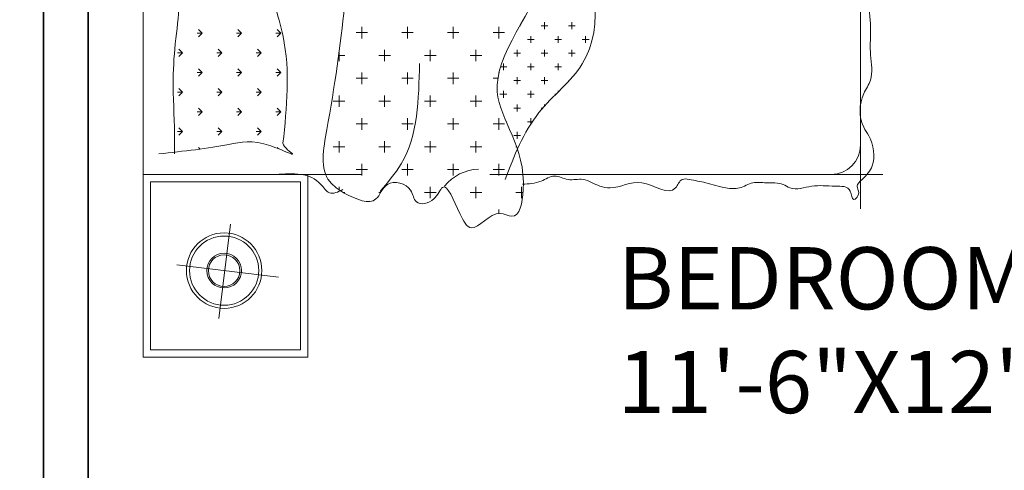
# Model space of a CAD drawing. Units: inches. Extents: x 3731 to 4318, y 1310 to 2388.
# Tile 35 of 57: x 3833 to 3943, y 2192 to 2243. Entities that reach past the tile are written whole.
import ezdxf

# ---------------------------------------------------------------- set-up
doc = ezdxf.new("R2010")
doc.units = ezdxf.units.IN
for name, color, linetype, lineweight in [('A-ANNO-DIMS', 2, 'Continuous', 18), ('A-AREA-IDEN', 7, 'Continuous', 18), ('A-FURN', 8, 'Continuous', 13), ('A-WALL', 7, 'Continuous', 35)]:
    doc.layers.add(name, color=color, linetype=linetype, lineweight=lineweight)
doc.styles.get("Standard").update_dxf_attribs({"font": 'arial.ttf'})
doc.dimstyles.get("Standard").update_dxf_attribs({"dimtxt": 0.18, "dimasz": 0.18, "dimexe": 0.18, "dimexo": 0.0625, "dimgap": 0.09, "dimtad": 0, "dimtih": 1, "dimtoh": 1, "dimdec": 4, "dimzin": 0, "dimdsep": 46, "dimtxsty": 'Standard', "dimcen": 0.09, "dimadec": 0, "dimazin": 0, "dimtfac": 1, "dimtdec": 4, "dimtofl": 0, "dimtmove": 0, "dimatfit": 3, "dimfxl": 1, "dimtolj": 1, "dimtzin": 0, "dimarcsym": 0})

# ---------------------------------------------------------------- blocks, each defined once
blk = doc.blocks.new('A$C200C7901')
for p, q in [((0, 1.8834), (0, 2.3334)), ((0.5, 2.3334), (0, 2.3334)), ((0.5, 2.3334), (0.5, 1.7369)), ((0.5, 2.3334), (0.5, 1.7369)), ((0.5, 2.3334), (2, 2.3334)), ((0.5701, 1.9635), (0.5733, 1.9666)), ((0.5701, 1.9635), (0.5733, 1.9666)), ((0.5, 1.8834), (0, 1.8834)), ((0.4504, 1.782), (0.4504, 1.7863)), ((0.4504, 1.782), (0.4504, 1.7863)), ((0.458, 1.7977), (0.466, 1.7977)), ((0.458, 1.7977), (0.466, 1.7977)), ((0.4504, 1.6834), (0.4504, 1.6883)), ((0.4504, 1.6834), (0.4504, 1.6883)), ((0.4656, 1.6727), (0.466, 1.6727)), ((0.4656, 1.6727), (0.466, 1.6727)), ((0.5597, 1.6727), (0.591, 1.6727)), ((0.5597, 1.6727), (0.591, 1.6727)), ((0.4504, 1.532), (0.4504, 1.5633)), ((0.4347, 1.5477), (0.466, 1.5477)), ((0.6847, 1.5477), (0.716, 1.5477)), ((0.4347, 1.4227), (0.466, 1.4227)), ((0.5, 1.3845), (0.5, 0.3086)), ((0.3931, 1.3602), (0.4035, 1.3602)), ((0.3931, 1.3602), (0.4035, 1.3602)), ((0.4972, 1.3602), (0.5285, 1.3602)), ((0.4972, 1.3602), (0.5285, 1.3602)), ((0.4347, 1.2977), (0.466, 1.2977)), ((0.4347, 1.2977), (0.466, 1.2977)), ((0.4504, 1.2936), (0.4504, 1.3133)), ((0.4504, 1.2936), (0.4504, 1.3133)), ((0.4061, 0.3703), (2.0386, 0.3703))]:
    blk.add_line(p, q)
at = {"linetype": 'ByBlock'}
for p, q in [((0.02, 1.9034), (0.02, 2.3134)), ((0.48, 2.3134), (0.02, 2.3134)), ((0.48, 1.9034), (0.48, 2.3134)), ((0.2524, 2.2412), (0.2186, 1.9635)), ((0.6171, 2.2259), (0.6171, 2.2402)), ((0.6171, 2.2259), (0.6171, 2.2402)), ((0.7249, 2.2259), (0.7249, 2.2402)), ((0.7249, 2.2259), (0.7249, 2.2402)), ((0.8326, 2.2259), (0.8326, 2.2402)), ((0.8326, 2.2259), (0.8326, 2.2402)), ((0.6171, 2.2259), (0.607, 2.236)), ((0.6171, 2.2259), (0.607, 2.236)), ((0.6171, 2.2259), (0.6272, 2.236)), ((0.6171, 2.2259), (0.6272, 2.236)), ((0.7249, 2.2259), (0.7148, 2.236)), ((0.7249, 2.2259), (0.7148, 2.236)), ((0.7249, 2.2259), (0.735, 2.236)), ((0.7249, 2.2259), (0.735, 2.236)), ((0.8326, 2.2259), (0.8225, 2.236)), ((0.8326, 2.2259), (0.8225, 2.236)), ((0.8326, 2.2259), (0.8427, 2.236)), ((0.8326, 2.2259), (0.8427, 2.236)), ((0.671, 2.172), (0.671, 2.1863)), ((0.671, 2.172), (0.671, 2.1863)), ((0.7787, 2.172), (0.7787, 2.1863)), ((0.7787, 2.172), (0.7787, 2.1863)), ((0.8865, 2.172), (0.8865, 2.1863)), ((0.8865, 2.172), (0.8865, 2.1863)), ((0.5692, 2.178), (0.5733, 2.1822)), ((0.5692, 2.178), (0.5733, 2.1822)), ((0.671, 2.1721), (0.6609, 2.1822)), ((0.671, 2.1721), (0.6609, 2.1822)), ((0.671, 2.1721), (0.6811, 2.1822)), ((0.671, 2.1721), (0.6811, 2.1822)), ((0.7787, 2.1721), (0.7686, 2.1822)), ((0.7787, 2.1721), (0.7686, 2.1822)), ((0.7787, 2.1721), (0.7889, 2.1822)), ((0.7787, 2.1721), (0.7889, 2.1822)), ((0.8865, 2.1721), (0.8764, 2.1822)), ((0.8865, 2.1721), (0.8764, 2.1822)), ((0.8865, 2.1721), (0.8966, 2.1822)), ((0.8865, 2.1721), (0.8966, 2.1822)), ((0.6171, 2.1182), (0.6171, 2.1325)), ((0.6171, 2.1182), (0.6171, 2.1325)), ((0.7249, 2.1182), (0.7249, 2.1325)), ((0.7249, 2.1182), (0.7249, 2.1325)), ((0.8326, 2.1182), (0.8326, 2.1325)), ((0.8326, 2.1182), (0.8326, 2.1325)), ((0.3641, 2.0951), (0.1061, 2.1268)), ((0.6171, 2.1182), (0.607, 2.1283)), ((0.6171, 2.1182), (0.607, 2.1283)), ((0.6171, 2.1182), (0.6272, 2.1283)), ((0.6171, 2.1182), (0.6272, 2.1283)), ((0.7249, 2.1182), (0.7148, 2.1283)), ((0.7249, 2.1182), (0.7148, 2.1283)), ((0.7249, 2.1182), (0.735, 2.1283)), ((0.7249, 2.1182), (0.735, 2.1283)), ((0.8326, 2.1182), (0.8225, 2.1283)), ((0.8326, 2.1182), (0.8225, 2.1283)), ((0.8326, 2.1182), (0.8427, 2.1283)), ((0.8326, 2.1182), (0.8427, 2.1283)), ((0.671, 2.0643), (0.671, 2.0786)), ((0.671, 2.0643), (0.671, 2.0786)), ((0.7787, 2.0643), (0.7787, 2.0786)), ((0.7787, 2.0643), (0.7787, 2.0786)), ((0.8865, 2.0643), (0.8865, 2.0786)), ((0.8865, 2.0643), (0.8865, 2.0786)), ((0.671, 2.0643), (0.6609, 2.0744)), ((0.671, 2.0643), (0.6609, 2.0744)), ((0.671, 2.0643), (0.6811, 2.0744)), ((0.671, 2.0643), (0.6811, 2.0744)), ((0.7787, 2.0643), (0.7686, 2.0744)), ((0.7787, 2.0643), (0.7686, 2.0744)), ((0.7787, 2.0643), (0.7889, 2.0744)), ((0.7787, 2.0643), (0.7889, 2.0744)), ((0.8865, 2.0643), (0.8764, 2.0744)), ((0.8865, 2.0643), (0.8764, 2.0744)), ((0.8865, 2.0643), (0.8966, 2.0744)), ((0.8865, 2.0643), (0.8966, 2.0744)), ((0.6171, 2.0104), (0.6171, 2.0247)), ((0.6171, 2.0104), (0.6171, 2.0247)), ((0.7249, 2.0104), (0.7249, 2.0247)), ((0.7249, 2.0104), (0.7249, 2.0247)), ((0.8326, 2.0104), (0.8326, 2.0247)), ((0.8326, 2.0104), (0.8326, 2.0247)), ((0.6171, 2.0104), (0.607, 2.0205)), ((0.6171, 2.0104), (0.607, 2.0205)), ((0.6171, 2.0104), (0.6272, 2.0205)), ((0.6171, 2.0104), (0.6272, 2.0205)), ((0.7249, 2.0104), (0.7148, 2.0205)), ((0.7249, 2.0104), (0.7148, 2.0205)), ((0.7249, 2.0104), (0.735, 2.0205)), ((0.7249, 2.0104), (0.735, 2.0205)), ((0.8326, 2.0104), (0.8225, 2.0205)), ((0.8326, 2.0104), (0.8225, 2.0205)), ((0.8326, 2.0104), (0.8427, 2.0205)), ((0.8326, 2.0104), (0.8427, 2.0205)), ((0.671, 1.9565), (0.671, 1.9708)), ((0.671, 1.9565), (0.671, 1.9708)), ((0.7787, 1.9565), (0.7787, 1.9708)), ((0.7787, 1.9565), (0.7787, 1.9708)), ((0.8865, 1.9565), (0.8865, 1.9708)), ((0.8865, 1.9565), (0.8865, 1.9708)), ((0.671, 1.9565), (0.6609, 1.9666)), ((0.671, 1.9565), (0.6609, 1.9666)), ((0.671, 1.9565), (0.6811, 1.9666)), ((0.671, 1.9565), (0.6811, 1.9666)), ((0.7787, 1.9565), (0.7686, 1.9666)), ((0.7787, 1.9565), (0.7686, 1.9666)), ((0.7787, 1.9565), (0.7889, 1.9666)), ((0.7787, 1.9565), (0.7889, 1.9666)), ((0.8865, 1.9565), (0.8764, 1.9666)), ((0.8865, 1.9565), (0.8764, 1.9666)), ((0.8865, 1.9565), (0.8966, 1.9666)), ((0.8865, 1.9565), (0.8966, 1.9666)), ((0.48, 1.9034), (0.02, 1.9034)), ((0.5754, 1.782), (0.5754, 1.8133)), ((0.5754, 1.782), (0.5754, 1.8133)), ((0.7004, 1.782), (0.7004, 1.8133)), ((0.7004, 1.782), (0.7004, 1.8133)), ((0.5597, 1.7977), (0.591, 1.7977)), ((0.5597, 1.7977), (0.591, 1.7977)), ((0.6847, 1.7977), (0.716, 1.7977)), ((0.6847, 1.7977), (0.716, 1.7977)), ((0.8097, 1.7977), (0.8331, 1.7977)), ((0.8097, 1.7977), (0.8331, 1.7977)), ((0.8254, 1.782), (0.8254, 1.7987)), ((0.8254, 1.782), (0.8254, 1.7987)), ((0.4972, 1.7352), (0.5285, 1.7352)), ((0.4972, 1.7352), (0.5285, 1.7352)), ((0.5129, 1.7195), (0.5129, 1.7508)), ((0.5129, 1.7195), (0.5129, 1.7508)), ((0.6222, 1.7352), (0.6535, 1.7352)), ((0.6222, 1.7352), (0.6535, 1.7352)), ((0.6379, 1.7195), (0.6379, 1.7508)), ((0.6379, 1.7195), (0.6379, 1.7508)), ((0.7472, 1.7352), (0.7785, 1.7352)), ((0.7472, 1.7352), (0.7785, 1.7352)), ((0.7629, 1.7195), (0.7629, 1.7508)), ((0.7629, 1.7195), (0.7629, 1.7508)), ((0.8722, 1.7352), (0.9035, 1.7352)), ((0.8722, 1.7352), (0.9035, 1.7352)), ((0.8879, 1.7195), (0.8879, 1.7508)), ((0.8879, 1.7195), (0.8879, 1.7508)), ((0.5754, 1.657), (0.5754, 1.6883)), ((0.5754, 1.657), (0.5754, 1.6883)), ((0.6847, 1.6727), (0.716, 1.6727)), ((0.6847, 1.6727), (0.716, 1.6727)), ((0.7004, 1.657), (0.7004, 1.6883)), ((0.7004, 1.657), (0.7004, 1.6883)), ((0.8097, 1.6727), (0.841, 1.6727)), ((0.8097, 1.6727), (0.841, 1.6727)), ((0.8254, 1.657), (0.8254, 1.6883)), ((0.8254, 1.657), (0.8254, 1.6883)), ((0.5129, 1.5945), (0.5129, 1.6258)), ((0.5129, 1.5945), (0.5129, 1.6258)), ((0.6379, 1.5945), (0.6379, 1.6258)), ((0.6379, 1.5945), (0.6379, 1.6258)), ((0.7629, 1.5945), (0.7629, 1.6258)), ((0.7629, 1.5945), (0.7629, 1.6258)), ((0.8879, 1.5945), (0.8879, 1.6258)), ((0.8879, 1.5945), (0.8879, 1.6258)), ((0.4972, 1.6102), (0.5285, 1.6102)), ((0.4972, 1.6102), (0.5285, 1.6102)), ((0.6222, 1.6102), (0.6535, 1.6102)), ((0.6222, 1.6102), (0.6535, 1.6102)), ((0.7472, 1.6102), (0.7785, 1.6102)), ((0.7472, 1.6102), (0.7785, 1.6102)), ((0.8722, 1.6102), (0.9035, 1.6102)), ((0.8722, 1.6102), (0.9035, 1.6102)), ((0.4504, 1.532), (0.4504, 1.5633)), ((0.5754, 1.532), (0.5754, 1.5633)), ((0.5754, 1.532), (0.5754, 1.5633)), ((0.7004, 1.532), (0.7004, 1.5633)), ((0.7004, 1.532), (0.7004, 1.5633)), ((0.8254, 1.532), (0.8254, 1.5633)), ((0.8254, 1.532), (0.8254, 1.5633)), ((0.4347, 1.5477), (0.466, 1.5477)), ((0.5597, 1.5477), (0.591, 1.5477)), ((0.5597, 1.5477), (0.591, 1.5477)), ((0.6847, 1.5477), (0.716, 1.5477)), ((0.8097, 1.5477), (0.841, 1.5477)), ((0.8097, 1.5477), (0.841, 1.5477)), ((0.4972, 1.4852), (0.5285, 1.4852)), ((0.4972, 1.4852), (0.5285, 1.4852)), ((0.5129, 1.4695), (0.5129, 1.5008)), ((0.5129, 1.4695), (0.5129, 1.5008)), ((0.6222, 1.4852), (0.6535, 1.4852)), ((0.6222, 1.4852), (0.6535, 1.4852)), ((0.6379, 1.4695), (0.6379, 1.5008)), ((0.6379, 1.4695), (0.6379, 1.5008)), ((0.7472, 1.4852), (0.7785, 1.4852)), ((0.7472, 1.4852), (0.7785, 1.4852)), ((0.7629, 1.4695), (0.7629, 1.5008)), ((0.7629, 1.4695), (0.7629, 1.5008)), ((0.8722, 1.4852), (0.9035, 1.4852)), ((0.8722, 1.4852), (0.9035, 1.4852)), ((0.8879, 1.4695), (0.8879, 1.5008)), ((0.8879, 1.4695), (0.8879, 1.5008)), ((0.4504, 1.407), (0.4504, 1.4383)), ((0.4504, 1.407), (0.4504, 1.4383)), ((0.5754, 1.407), (0.5754, 1.4383)), ((0.5754, 1.407), (0.5754, 1.4383)), ((0.7004, 1.407), (0.7004, 1.4383)), ((0.7004, 1.407), (0.7004, 1.4383)), ((0.8254, 1.407), (0.8254, 1.4383)), ((0.8254, 1.407), (0.8254, 1.4383)), ((0.4347, 1.4227), (0.466, 1.4227)), ((0.5597, 1.4227), (0.591, 1.4227)), ((0.5597, 1.4227), (0.591, 1.4227)), ((0.6847, 1.4227), (0.716, 1.4227)), ((0.6847, 1.4227), (0.716, 1.4227)), ((0.8097, 1.4227), (0.841, 1.4227)), ((0.8097, 1.4227), (0.841, 1.4227)), ((0.5129, 1.3445), (0.5129, 1.3758)), ((0.5129, 1.3445), (0.5129, 1.3758)), ((0.6379, 1.3445), (0.6379, 1.3758)), ((0.6379, 1.3445), (0.6379, 1.3758)), ((0.7629, 1.3627), (0.7629, 1.3758)), ((0.7629, 1.3627), (0.7629, 1.3758)), ((0.8879, 1.3445), (0.8879, 1.3758)), ((0.8879, 1.3445), (0.8879, 1.3758)), ((0.6222, 1.3602), (0.6535, 1.3602)), ((0.6222, 1.3602), (0.6535, 1.3602)), ((0.7097, 1.3477), (0.7285, 1.3477)), ((0.7097, 1.3477), (0.7285, 1.3477)), ((0.7191, 1.3383), (0.7191, 1.357)), ((0.7191, 1.3383), (0.7191, 1.357)), ((0.7762, 1.3602), (0.7785, 1.3602)), ((0.7762, 1.3602), (0.7785, 1.3602)), ((0.7847, 1.3477), (0.8035, 1.3477)), ((0.7847, 1.3477), (0.8035, 1.3477)), ((0.7941, 1.3383), (0.7941, 1.3554)), ((0.7941, 1.3383), (0.7941, 1.3554)), ((0.8722, 1.3602), (0.9035, 1.3602)), ((0.8722, 1.3602), (0.9035, 1.3602)), ((0.6441, 1.3383), (0.6441, 1.3399)), ((0.6441, 1.3383), (0.6441, 1.3399)), ((0.5754, 1.3115), (0.5754, 1.3133)), ((0.5754, 1.3115), (0.5754, 1.3133)), ((0.5972, 1.3102), (0.616, 1.3102)), ((0.5972, 1.3102), (0.616, 1.3102)), ((0.6066, 1.3008), (0.6066, 1.3195)), ((0.6066, 1.3008), (0.6066, 1.3195)), ((0.6722, 1.3102), (0.691, 1.3102)), ((0.6722, 1.3102), (0.691, 1.3102)), ((0.6816, 1.3008), (0.6816, 1.3195)), ((0.6816, 1.3008), (0.6816, 1.3195)), ((0.7472, 1.3102), (0.766, 1.3102)), ((0.7472, 1.3102), (0.766, 1.3102)), ((0.7566, 1.3008), (0.7566, 1.3195)), ((0.7566, 1.3008), (0.7566, 1.3195)), ((0.8222, 1.3102), (0.841, 1.3102)), ((0.8222, 1.3102), (0.841, 1.3102)), ((0.8316, 1.3008), (0.8316, 1.3195)), ((0.8316, 1.3008), (0.8316, 1.3195)), ((0.9066, 1.3008), (0.9066, 1.3028)), ((0.9066, 1.3008), (0.9066, 1.3028)), ((0.6379, 1.2727), (0.6535, 1.2727)), ((0.6379, 1.2727), (0.6535, 1.2727)), ((0.6441, 1.2686), (0.6441, 1.282)), ((0.6441, 1.2686), (0.6441, 1.282)), ((0.7097, 1.2727), (0.7285, 1.2727)), ((0.7097, 1.2727), (0.7285, 1.2727)), ((0.7191, 1.2633), (0.7191, 1.282)), ((0.7191, 1.2633), (0.7191, 1.282)), ((0.7847, 1.2727), (0.8035, 1.2727)), ((0.7847, 1.2727), (0.8035, 1.2727)), ((0.7941, 1.2633), (0.7941, 1.282)), ((0.7941, 1.2633), (0.7941, 1.282)), ((0.8597, 1.2727), (0.8785, 1.2727)), ((0.8597, 1.2727), (0.8785, 1.2727)), ((0.8691, 1.2633), (0.8691, 1.282)), ((0.8691, 1.2633), (0.8691, 1.282)), ((0.6816, 1.2398), (0.6816, 1.2445)), ((0.6816, 1.2398), (0.6816, 1.2445)), ((0.7566, 1.2258), (0.7566, 1.2445)), ((0.7566, 1.2258), (0.7566, 1.2445)), ((0.8316, 1.2258), (0.8316, 1.2445)), ((0.8316, 1.2258), (0.8316, 1.2445)), ((0.9066, 1.2258), (0.9066, 1.2445)), ((0.9066, 1.2258), (0.9066, 1.2445)), ((0.6868, 1.2352), (0.691, 1.2352)), ((0.6868, 1.2352), (0.691, 1.2352)), ((0.7472, 1.2352), (0.766, 1.2352)), ((0.7472, 1.2352), (0.766, 1.2352)), ((0.8222, 1.2352), (0.841, 1.2352)), ((0.8222, 1.2352), (0.841, 1.2352)), ((0.8972, 1.2352), (0.916, 1.2352)), ((0.8972, 1.2352), (0.916, 1.2352)), ((0.7191, 1.2041), (0.7191, 1.207)), ((0.7191, 1.2041), (0.7191, 1.207)), ((0.7255, 1.1977), (0.7285, 1.1977)), ((0.7255, 1.1977), (0.7285, 1.1977)), ((0.7847, 1.1977), (0.8035, 1.1977)), ((0.7847, 1.1977), (0.8035, 1.1977)), ((0.7941, 1.1883), (0.7941, 1.207)), ((0.7941, 1.1883), (0.7941, 1.207)), ((0.8597, 1.1977), (0.8785, 1.1977)), ((0.8597, 1.1977), (0.8785, 1.1977)), ((0.8691, 1.1883), (0.8691, 1.207)), ((0.8691, 1.1883), (0.8691, 1.207)), ((0.7566, 1.1674), (0.7566, 1.1695)), ((0.7566, 1.1674), (0.7566, 1.1695)), ((0.7646, 1.1602), (0.766, 1.1602)), ((0.7646, 1.1602), (0.766, 1.1602)), ((0.8222, 1.1602), (0.841, 1.1602)), ((0.8222, 1.1602), (0.841, 1.1602)), ((0.8316, 1.1508), (0.8316, 1.1695)), ((0.8316, 1.1508), (0.8316, 1.1695)), ((0.8972, 1.1602), (0.916, 1.1602)), ((0.8972, 1.1602), (0.916, 1.1602)), ((0.9066, 1.1508), (0.9066, 1.1695)), ((0.9066, 1.1508), (0.9066, 1.1695)), ((0.8691, 1.1133), (0.8691, 1.132)), ((0.8691, 1.1133), (0.8691, 1.132)), ((0.8597, 1.1227), (0.8785, 1.1227)), ((0.8597, 1.1227), (0.8785, 1.1227))]:
    blk.add_line(p, q, dxfattribs=at)
for radius in [0.1032, 0.0947, 0.0475, 0.0432]:
    blk.add_circle((0.2367, 2.1121), radius, dxfattribs=at)
blk.add_arc((0.3888, 1.4113), 0.1256, 1.9962, 51.1646, dxfattribs=at)
for centre, radius, start, end in [((0.3888, 1.4113), 0.1256, 1.9962, 51.1646), ((0.58, 0.4503), 0.08, 180, 270)]:
    blk.add_arc(centre, radius, start, end)
for points, knots in [([(0.5562, 2.2908), (0.5634, 2.223), (0.5751, 2.1147), (0.6005, 2.0213), (0.5392, 1.8966), (0.5726, 1.9486), (0.5854, 1.951)], [0, 0, 0, 0, 193.119101, 308.278592, 371.468985, 410.593498, 410.593498, 410.593498, 410.593498]), ([(0.5854, 1.951), (0.6835, 1.9407), (0.8425, 1.9242), (1.0374, 2.0054), (1.1564, 1.9255), (1.2274, 1.9841), (1.2052, 2.0751), (1.1815, 2.152), (1.2176, 2.2368), (1.0992, 2.2731), (1.0008, 2.2255), (0.8698, 2.246), (0.7481, 2.2548), (0.6426, 2.2473), (0.5746, 2.2478), (0.5562, 2.2479)], [0, 0, 0, 0, 292.165466, 473.33038, 601.631673, 630.723769, 727.138505, 836.819956, 887.958136, 954.42438, 1118.989809, 1227.016542, 1338.750986, 1487.447361, 1542.751028, 1542.751028, 1542.751028, 1542.751028]), ([(0.4485, 1.7835), (0.4321, 1.7496), (0.4062, 1.6964), (0.49, 1.6713), (0.4719, 1.5969), (0.4123, 1.592), (0.4233, 1.5337), (0.4954, 1.5086), (0.4012, 1.4738), (0.3253, 1.4306), (0.4113, 1.3764), (0.3688, 1.3065), (0.5579, 1.2663), (0.741, 1.4533), (1.1127, 1.1109), (1.4811, 1.2478), (1.7885, 1.3492), (2.0357, 1.1637), (2.0748, 1.2974), (2.0876, 1.349), (2.0192, 1.3805), (2.0564, 1.4298), (2.0588, 1.4846), (1.9759, 1.5349), (2.1004, 1.5845), (2.0397, 1.6519), (1.971, 1.7053), (2.1104, 1.8981), (1.5946, 1.7967), (1.2448, 1.7472), (0.8129, 1.7935), (0.4953, 1.8548), (0.4582, 1.7983), (0.4485, 1.7835)], [0, 0, 0, 0, 88.420092, 139.08588, 204.302936, 239.695496, 287.801042, 327.365471, 412.960499, 463.626286, 552.059846, 584.668336, 662.614915, 940.993281, 1309.926334, 1844.022653, 1996.276242, 2316.43048, 2341.441004, 2404.707416, 2449.463774, 2514.680778, 2538.40571, 2613.031547, 2697.13096, 2760.903931, 2822.692699, 2945.47, 3215.060018, 3725.584917, 4361.974444, 4504.671998, 4555.32777, 4555.32777, 4555.32777, 4555.32777]), ([(0.4856, 1.3429), (0.5504, 1.3182), (0.6715, 1.2721), (0.8374, 1.0498), (1.1164, 1.1183), (1.3878, 1.1816), (1.5888, 1.1102), (1.8403, 1.1127), (1.9415, 1.2178), (2.0032, 1.2819)], [0, 0, 0, 0, 205.411753, 383.654933, 772.067458, 921.644661, 1226.793228, 1388.983508, 1642.292305, 1642.292305, 1642.292305, 1642.292305])]:
    blk.add_open_spline(points, degree=3, knots=knots)
for points, knots in [([(0.5, 1.9703), (0.5029, 1.9235), (0.5066, 1.8648), (0.4398, 1.8252), (0.452, 1.8005), (0.4585, 1.7872)], [0, 0, 0, 0, 126.315232, 158.854004, 196.789047, 196.789047, 196.789047, 196.789047]), ([(0.5, 1.9703), (0.5029, 1.9235), (0.5066, 1.8648), (0.4398, 1.8252), (0.452, 1.8005), (0.4585, 1.7872)], [0, 0, 0, 0, 126.315232, 158.854004, 196.789047, 196.789047, 196.789047, 196.789047]), ([(0.4532, 1.6853), (0.4776, 1.6644), (0.574, 1.582), (0.7055, 1.5794), (0.8037, 1.5774)], [0, 0, 0, 0, 94.920667, 374.457292, 374.457292, 374.457292, 374.457292]), ([(0.4532, 1.6853), (0.4776, 1.6644), (0.574, 1.582), (0.7055, 1.5794), (0.8037, 1.5774)], [0, 0, 0, 0, 94.920667, 374.457292, 374.457292, 374.457292, 374.457292]), ([(0.473, 1.2954), (0.4739, 1.2781), (0.4755, 1.2477), (0.5032, 1.2084), (0.4801, 1.1701), (0.4928, 1.1255), (0.4674, 1.0912), (0.4579, 1.0351), (0.501, 0.9724), (0.4311, 0.8832), (0.4902, 0.8637), (0.4843, 0.8288), (0.4774, 0.7906), (0.4625, 0.7457), (0.459, 0.6999), (0.4816, 0.6664), (0.4748, 0.625), (0.4791, 0.5889), (0.4533, 0.5528), (0.4738, 0.5004), (0.4658, 0.4502), (0.4696, 0.3946), (0.4189, 0.3935), (0.4493, 0.3684), (0.4694, 0.3857), (0.4922, 0.3576), (0.5297, 0.3262), (0.5917, 0.3353), (0.6454, 0.3754), (0.7083, 0.3741), (0.7643, 0.3328), (0.826, 0.346), (0.925, 0.3388), (1.0353, 0.3593), (1.1561, 0.3744), (1.2477, 0.3154), (1.3302, 0.3474), (1.4086, 0.3512), (1.5217, 0.3878), (1.6362, 0.3176), (1.7682, 0.3285), (1.8402, 0.3019), (1.9071, 0.3529), (1.9647, 0.3412), (2.0795, 0.2948), (2.0472, 0.3498), (2.0343, 0.3772), (2.0435, 0.43), (2.0109, 0.5782), (2.0746, 0.4643), (2.0805, 0.584), (2.0084, 0.5979), (2.0343, 0.6846), (2.0344, 0.746), (2.0293, 0.8096), (2.0489, 0.8545), (2.0652, 0.9218), (1.9842, 0.9297), (2.0007, 1.0162), (2.0367, 1.0585), (2.0367, 1.1102), (2.0457, 1.1647), (2.0226, 1.2084), (2.0234, 1.2306), (2.0236, 1.2352)], [0, 0, 0, 0, 51.660678, 90.967412, 128.902454, 170.303599, 219.852997, 247.834962, 336.321557, 429.35469, 458.821847, 477.222321, 524.135809, 581.038434, 617.839381, 657.146115, 693.947125, 740.178081, 760.753248, 820.731705, 885.133458, 928.777044, 953.563729, 976.574207, 995.553042, 1018.563482, 1064.584401, 1147.951297, 1174.787598, 1266.851571, 1308.018447, 1377.066427, 1441.511314, 1608.245014, 1714.11869, 1792.771707, 1913.247991, 1954.931389, 2029.864445, 2259.189419, 2305.221512, 2429.507982, 2456.344283, 2543.92595, 2627.925037, 2662.96218, 2687.736879, 2719.937755, 2839.540991, 2875.47895, 2953.681041, 2993.270313, 3066.872333, 3154.395764, 3200.397042, 3248.426375, 3312.828127, 3347.881398, 3444.484026, 3481.577522, 3518.665244, 3592.267265, 3644.719162, 3658.519501, 3658.519501, 3658.519501, 3658.519501])]:
    blk.add_open_spline(points, degree=3, knots=knots, dxfattribs=at)
blk = doc.blocks.new('*D33')
at = {"layer": 'A-ANNO-DIMS', "color": 0, "lineweight": -2, "transparency": 16777216}
for p, q in [((3835.15, 2338.38), (3731.41, 2338.38)), ((3731.59, 2338.2), (3731.59, 1849.06)), ((3731.59, 1359.56), (3731.59, 1848.7)), ((3835.15, 1359.38), (3731.41, 1359.38))]:
    blk.add_line(p, q, dxfattribs=at)
at = {"layer": 'A-ANNO-DIMS', "color": 0, "transparency": 16777216}
for points in [[(3731.56, 2338.2), (3731.62, 2338.2), (3731.59, 2338.38)], [(3731.56, 1359.56), (3731.62, 1359.56), (3731.59, 1359.38)]]:
    blk.add_solid(points, dxfattribs=at)
at = {"layer": 'Defpoints', "color": 0, "transparency": 16777216}
for p in [(3731.59, 2338.38), (3835.21, 2338.38), (3835.21, 1359.38)]:
    blk.add_point(p, dxfattribs=at)
at = {"layer": 'A-ANNO-DIMS', "color": 0, "transparency": 16777216, "insert": (3731.59, 1848.88), "char_height": 0.18, "attachment_point": 5}
blk.add_mtext('\\A1;979', dxfattribs=at)

msp = doc.modelspace()

# ---------------------------------------------------------------- linework, layer by layer
at = {"layer": 'A-WALL'}
for p, q in [((3835.21, 2338.38), (3835.21, 1359.38)), ((3840.21, 2333.38), (3840.21, 2156.38))]:
    msp.add_line(p, q, dxfattribs=at)

# ---------------------------------------------------------------- block references
at = {"layer": 'A-FURN', "xscale": 41.1071563136412, "yscale": 41.1071563136412, "zscale": 41.1071563136412, "rotation": 90}
msp.add_blockref('A$C200C7901', (3942.35, 2204.6), dxfattribs=at)

# ---------------------------------------------------------------- texts
at = {"layer": 'A-AREA-IDEN', "insert": (3899.81, 2216.97), "char_height": 7, "attachment_point": 1}
msp.add_mtext_dynamic_manual_height_columns('BEDROOM\\P11\'-6"X12\'-6"', width=47.0437, gutter_width=12.5, heights=[0], dxfattribs=at)

# ---------------------------------------------------------------- dimensions: what is measured, and where the dimension line sits
at = {"layer": 'A-ANNO-DIMS'}
dim = msp.add_linear_dim(base=(3731.59, 2338.38), p1=(3835.21, 1359.38), p2=(3835.21, 2338.38), angle=90, dimstyle='Standard', override={"dimdec": 0, "dimlfac": 1, "dimrnd": 0, "dimzin": 0, "dimdsep": 46, "dimlunit": 2}, dxfattribs=at)
dim.commit()
dim.dimension.update_dxf_attribs({"geometry": '*D33', "text_midpoint": (3731.59, 1848.88)})

doc.saveas('drawing.dxf')
